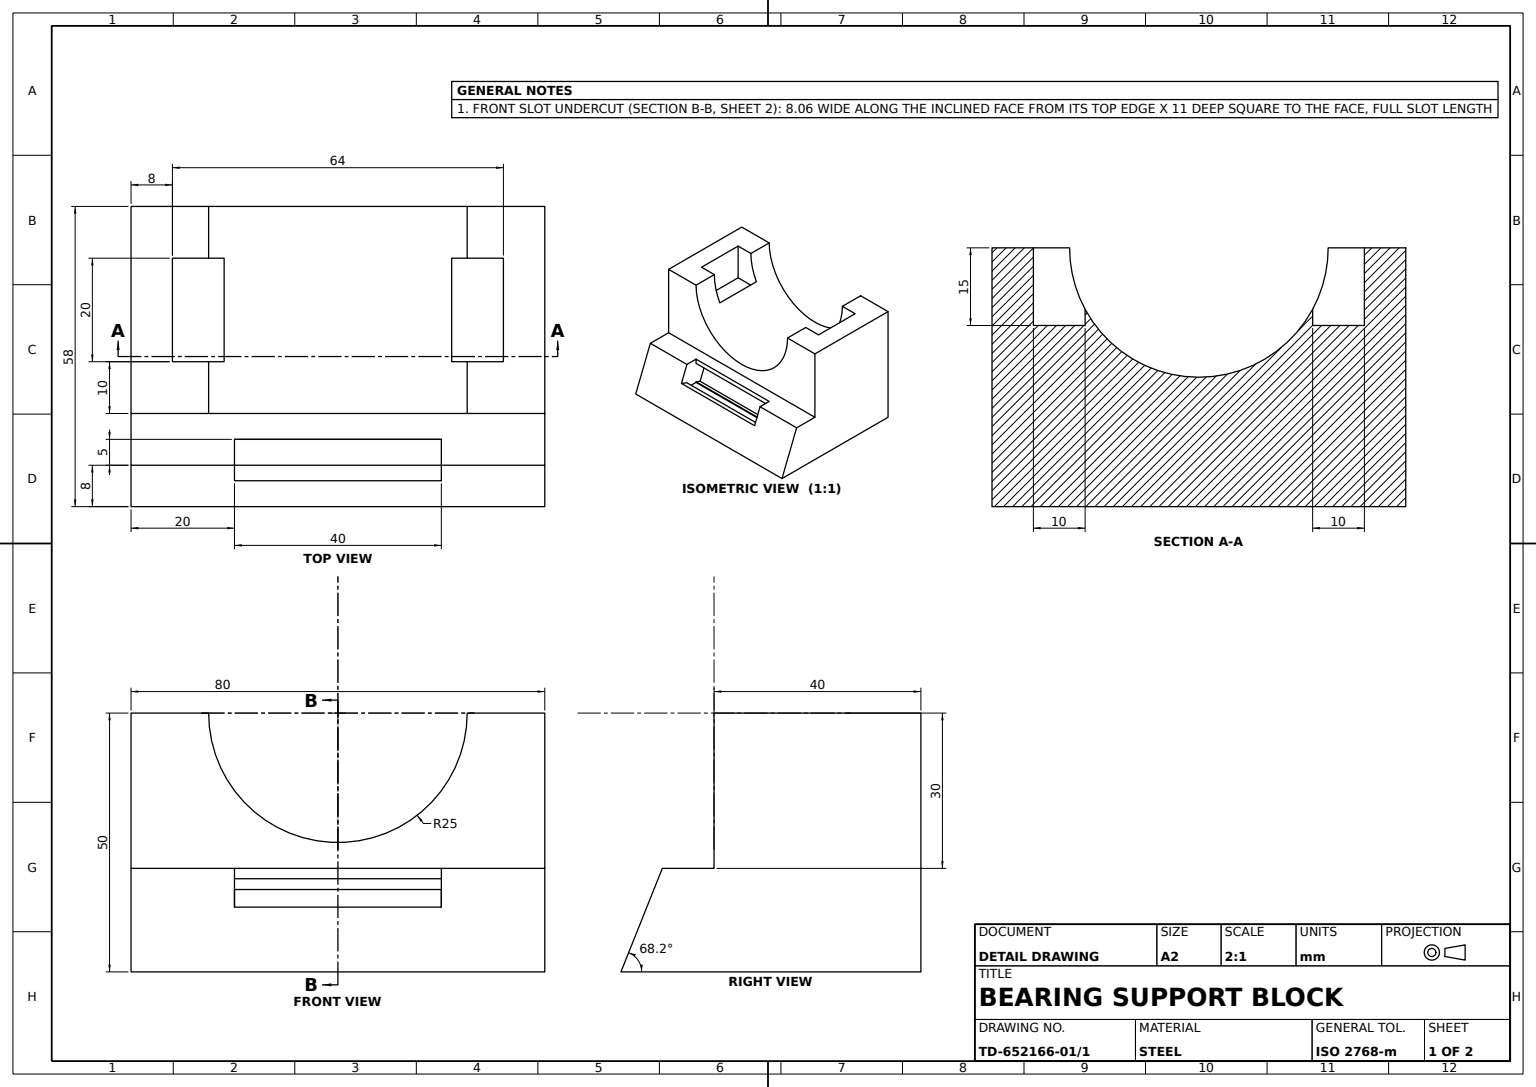
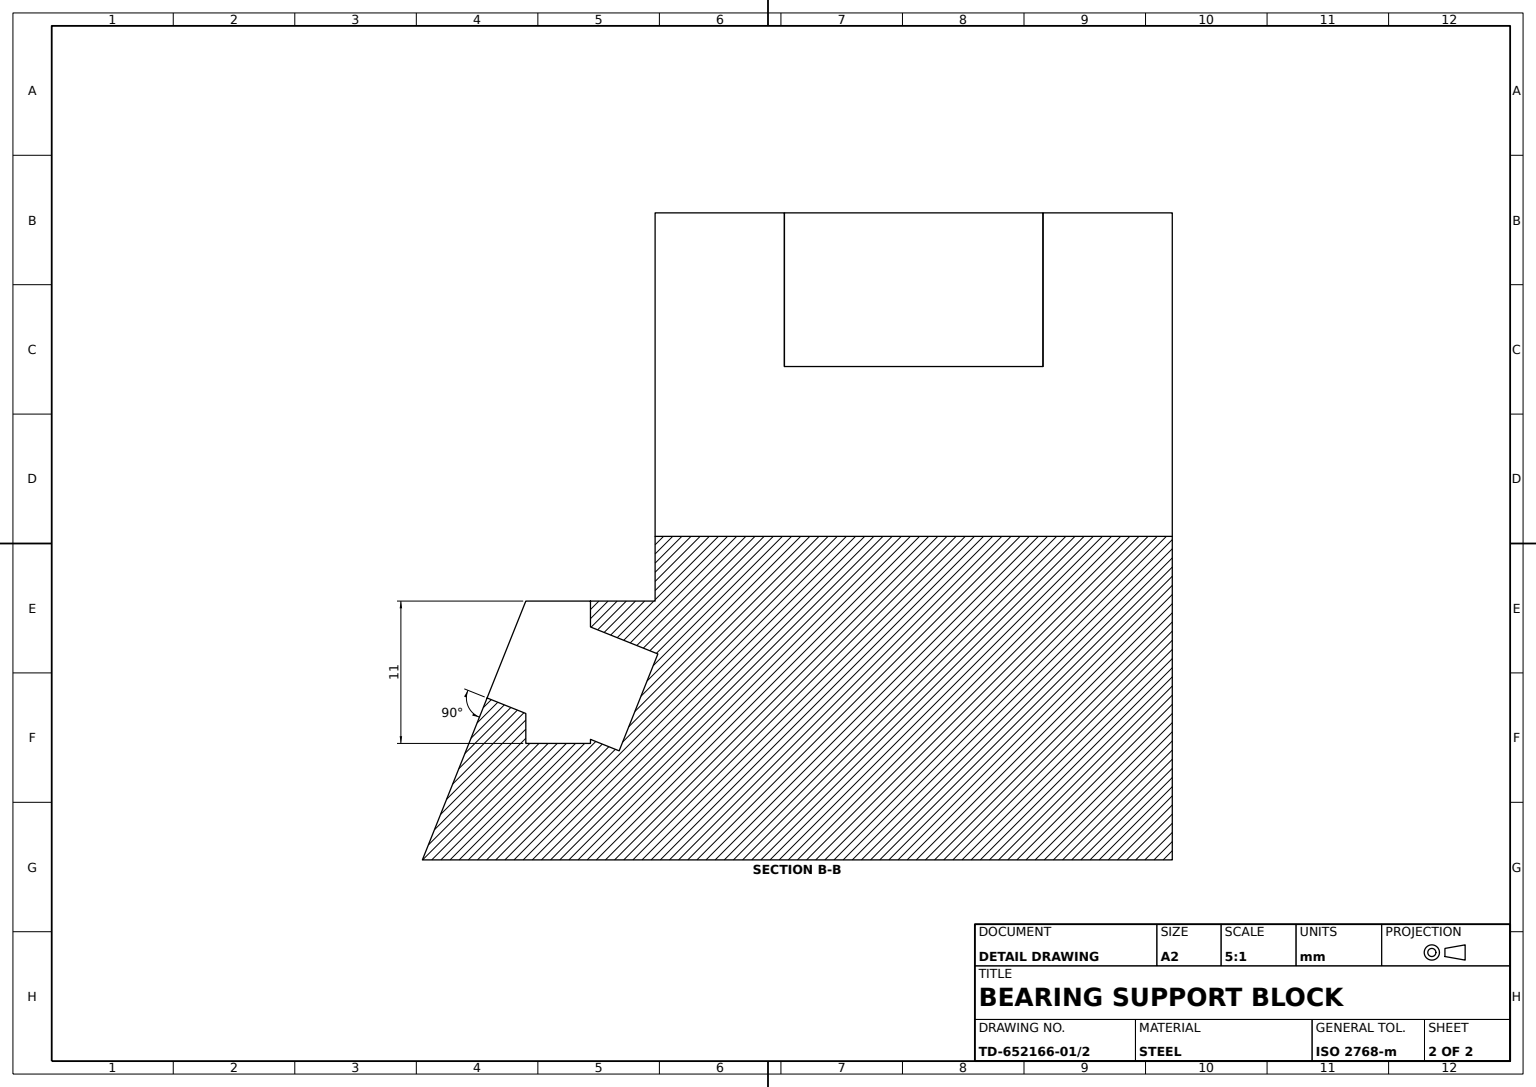
SolidWorks part; units mm, degrees
material "Plain Carbon Steel"
ref_plane "Front Plane" through (0, 0, 0) normal (0, 0, 1) x (1, 0, 0)
ref_plane "Top Plane" through (0, 0, 0) normal (0, 1, 0) x (1, 0, 0)
ref_plane "Right Plane" through (0, 0, 0) normal (1, 0, 0) x (0, 0, -1)
sketch "Base Profile Sketch" plane through (0, 0, 0) normal (0, 0, 1) x (1, 0, 0)
  line L0 (0, 0) -> (0, 50)
  line L1 (0, 50) -> (40, 50)
  line L2 (40, 50) -> (40, 20)
  line L3 (40, 20) -> (58, 20)
  line L4 (58, 20) -> (58, 0)
  line L5 (58, 0) -> (0, 0)
  dimension "D1" = 58
  dimension "D2" = 50
  dimension "D3" = 30
  dimension "D4" = 40
extrude "Base Block" add sketch "Base Profile Sketch" along normal blind 80
sketch "Upright Notches Sketch" plane through (0, 50, 0) normal (0, 1, 0) x (1, 0, 0)
  line L0 (10, -18) -> (10, -8)
  line L1 (10, -8) -> (30, -8)
  line L2 (30, -8) -> (30, -18)
  line L3 (30, -18) -> (10, -18)
  line L4 (0, -80) -> (0, 0) construction
  line L5 (10, -62) -> (10, -72)
  line L6 (10, -72) -> (30, -72)
  line L7 (30, -72) -> (30, -62)
  line L8 (30, -62) -> (10, -62)
  line L9 (40, -80) -> (0, -80) construction
  dimension "D1" = 20
  dimension "D2" = 10
  dimension "D3" = 20
  dimension "D4" = 8
  dimension "D5" = 64
  dimension "D6" = 10
  dimension "D7" = 10
extrude "Upright Top Notches" cut sketch "Upright Notches Sketch" against normal blind 15
sketch "Saddle Bore Sketch" plane through (40, 0, 0) normal (1, 0, 0) x (0, 0, -1)
  line L0 (-80, 50) -> (0, 50) construction
  circle A0 centre (-40, 50) radius 25
  dimension "D1" = 50
extrude "Saddle Bore Ø50" cut sketch "Saddle Bore Sketch" against normal through all
sketch "Front Slope Sketch" plane through (0, 0, 80) normal (0, 0, 1) x (1, 0, 0)
  line L0 (50, 20) -> (58, 20)
  line L1 (58, 0) -> (50, 20)
  line L2 (58, 20) -> (40, 20) construction
  line L3 (58, 20) -> (58, 0)
  dimension "D1" = 8
extrude "Front Slope Cut" cut sketch "Front Slope Sketch" against normal through all
sketch "Front Slot Sketch" plane through (0, 20, 0) normal (0, 1, 0) x (1, 0, 0)
  line L0 (50, -20) -> (45, -20)
  line L1 (50, 0) -> (50, -80) construction
  line L2 (45, -20) -> (45, -60)
  line L3 (45, -60) -> (50, -60)
  line L4 (50, -60) -> (50, -20)
  line L6 (40, -65) -> (40, -15) construction
  point P6 (40, -40)
  point P11 (50, -40)
  dimension "D1" = 5
  dimension "D2" = 40
extrude "Front Slot 40x5" cut sketch "Front Slot Sketch" against normal blind 11
sketch "Front Slot Undercut Sketch" plane through (50, 20, 0) normal (0.9285, 0.3714, 0) x (0, 0, -1)
  line L0 (-60, 0) -> (-60, -8.0643)
  line L1 (-60, -8.0643) -> (-20, -8.0643)
  line L2 (-20, -8.0643) -> (-20, 0)
  line L3 (-20, 0) -> (-60, 0)
  dimension "D1" = 8.0643
extrude "Front Slot Undercut" cut sketch "Front Slot Undercut Sketch" against normal blind 11
